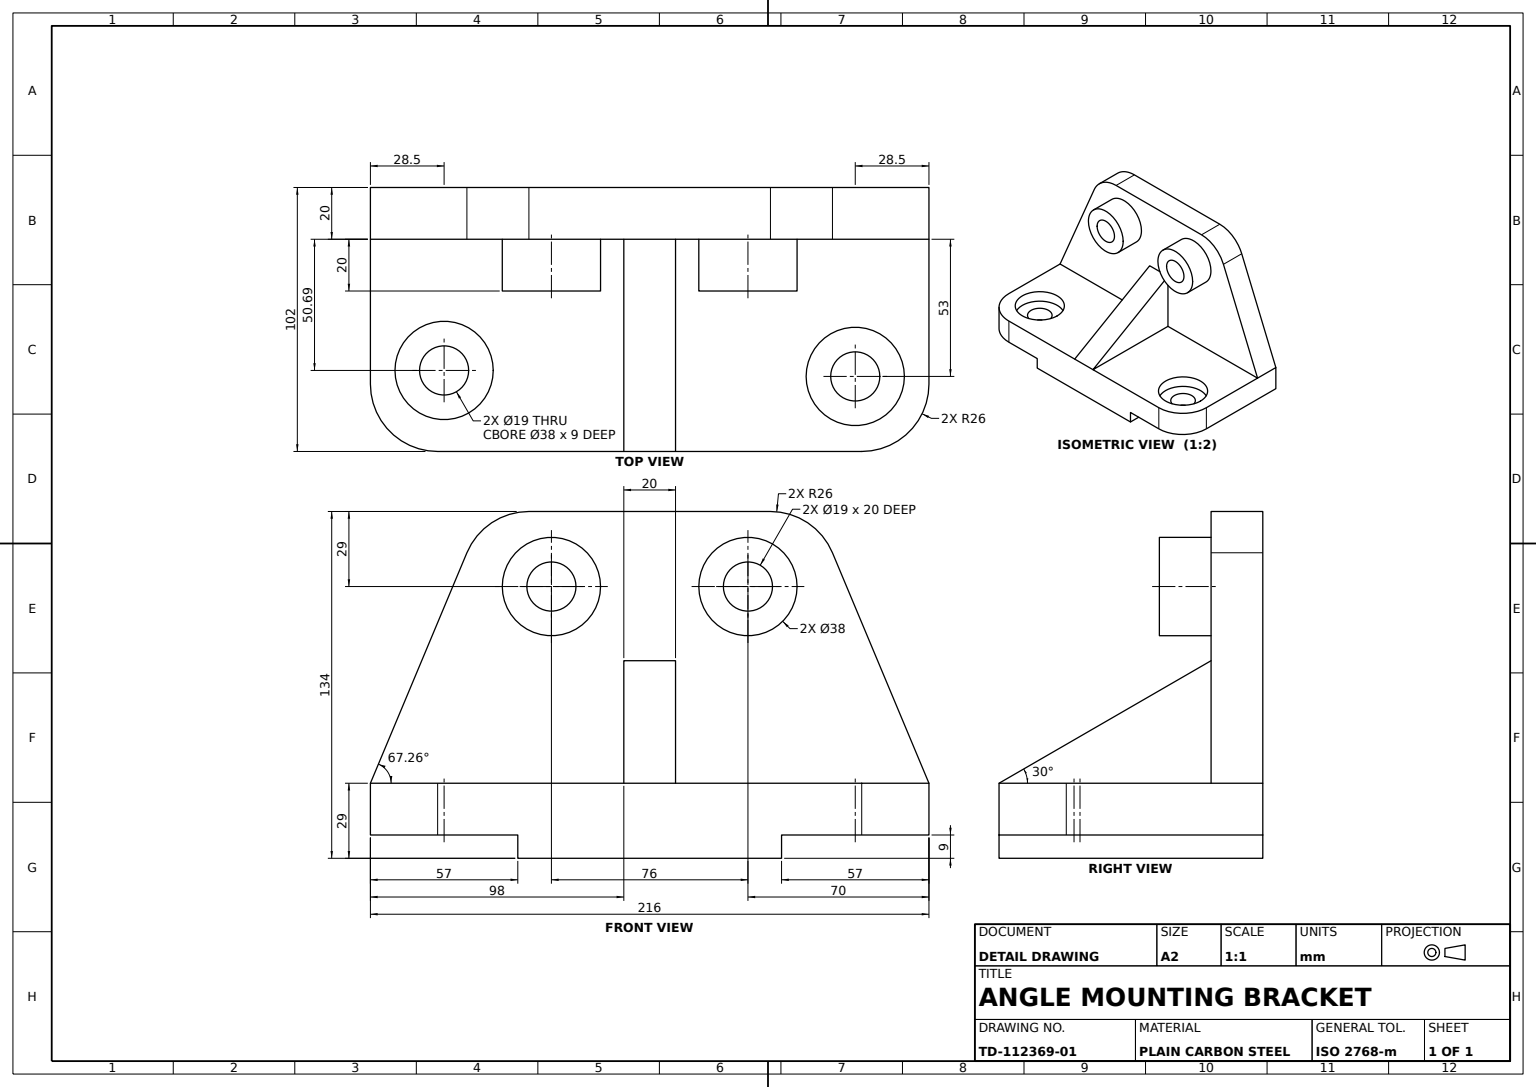
SolidWorks part; units mm, degrees
material "Plain Carbon Steel"
ref_plane "Front Plane" through (0, 0, 0) normal (0, 0, 1) x (1, 0, 0)
ref_plane "Top Plane" through (0, 0, 0) normal (0, 1, 0) x (1, 0, 0)
ref_plane "Right Plane" through (0, 0, 0) normal (1, 0, 0) x (0, 0, -1)
sketch "Base Plate Profile" plane through (0, 0, 0) normal (1, 0, 0) x (0, 0, -1)
  line L0 (0, 0) -> (57, 0)
  line L1 (57, 0) -> (57, -9)
  line L2 (57, -9) -> (159, -9)
  line L3 (159, -9) -> (159, 0)
  line L4 (159, 0) -> (216, 0)
  line L5 (216, 0) -> (216, 20)
  line L6 (216, 20) -> (0, 20)
  line L7 (0, 20) -> (0, 0)
  dimension "D1" = 57
  dimension "D2" = 9
  dimension "D3" = 102
  dimension "D4" = 216
  dimension "D5" = 20
extrude "Base Plate" add sketch "Base Plate Profile" along normal blind 102
ref_plane "Plane1" through (0, 0, 0) normal (1, 0, 0) x (0, 0, -1)
sketch "Upright Plate Profile" plane through (0, 0, 0) normal (1, 0, 0) x (0, 0, -1)
  line L0 (0, 20) -> (216, 20)
  line L2 (44, 125) -> (172, 125)
  line L4 (172, 125) -> (216, 20)
  line L5 (44, 125) -> (0, 20)
  dimension "D1" = 128
  dimension "D2" = 125
  dimension "D3" = 44
extrude "Upright Plate" add sketch "Upright Plate Profile" along normal blind 20
sketch "Upright Boss 1 Profile" plane through (20, 0, 0) normal (1, 0, 0) x (0, 0, -1)
  line L0 (172, 125) -> (44, 125) construction
  circle A0 centre (70, 96) radius 19
  circle A1 centre (70, 96) radius 9.5
  point P6 (108, 125)
  dimension "D1" = 76
  dimension "D3" = 19
  dimension "D4" = 38
  dimension "D2" = 38
extrude "Upright Boss 1" add sketch "Upright Boss 1 Profile" along normal blind 20
sketch "Upright Boss 2 Profile" plane through (20, 0, 0) normal (1, 0, 0) x (0, 0, -1)
  line L0 (0, 20) -> (216, 20) construction
  line L1 (172, 125) -> (44, 125) construction
  circle A0 centre (146, 96) radius 19
  circle A1 centre (146, 96) radius 9.5
  point P7 (108, 125)
  dimension "D1" = 76
  dimension "D3" = 19
  dimension "D4" = 38
  dimension "D2" = 38
extrude "Upright Boss 2" add sketch "Upright Boss 2 Profile" along normal blind 20
sketch "Base Pocket 1 Profile" plane through (0, 20, 0) normal (0, 1, 0) x (1, 0, 0)
  line L0 (102, 108) -> (102, 187.5) construction
  line L1 (102, 216) -> (102, 0) construction
  line L2 (102, 187.5) -> (73, 187.5) construction
  line L3 (73, 187.5) -> (73, 0) construction
  line L4 (102, 0) -> (20, 0) construction
  line L5 (102, 108) -> (102, 28.5) construction
  line L6 (102, 28.5) -> (73, 28.5) construction
  line L7 (20, 0) -> (20, 216) construction
  circle A0 centre (73, 187.5) radius 19
  dimension "D1" = 38
  dimension "D2" = 53
  dimension "D3" = 28.5
extrude "Base Pocket 1" cut sketch "Base Pocket 1 Profile" against normal blind 9
sketch "Mounting Hole 1 Profile" plane through (0, 11, 0) normal (0, 1, 0) x (1, 0, 0)
  circle A0 centre (73, 187.5) radius 9.5
  dimension "D1" = 19
extrude "Mounting Hole 1" cut sketch "Mounting Hole 1 Profile" against normal through all
sketch "Base Pocket 2 Profile" plane through (0, 20, 0) normal (0, 1, 0) x (1, 0, 0)
  line L0 (102, 108) -> (102, 28.5) construction
  line L1 (102, 216) -> (102, 0) construction
  line L2 (102, 28.5) -> (70.69, 28.5) construction
  line L3 (20, 0) -> (20, 216) construction
  circle A0 centre (70.69, 28.5) radius 19
  dimension "D1" = 38
  dimension "D2" = 50.69
  dimension "D3" = 28.5
extrude "Base Pocket 2" cut sketch "Base Pocket 2 Profile" against normal blind 9
sketch "Mounting Hole 2 Profile" plane through (0, 11, 0) normal (0, 1, 0) x (1, 0, 0)
  circle A0 centre (70.69, 28.5) radius 9.5
  dimension "D1" = 19
extrude "Mounting Hole 2" cut sketch "Mounting Hole 2 Profile" against normal through all
fillet "Upright Corner Fillet R26 1" radius 26 1 edges at (10, 125, -44)
fillet "Upright Corner Fillet R26 2" radius 26 1 edges at (10, 125, -172)
fillet "Base Corner Fillets R26" radius 26 2 edges at (102, 10, -216) (102, 10, 0)
ref_plane "Plane2" through (0, 0, -108) normal (0, 0, 1) x (1, 0, 0)
sketch "Gusset Rib Profile 30deg" plane through (0, 0, -108) normal (0, 0, 1) x (1, 0, 0)
  line L0 (102, 20) -> (20, 67.3427)
  line L1 (20, 109.0486) -> (20, 20) construction
  line L2 (102, 20) -> (76, 20) construction
  dimension "D1" = 30
rib "Gusset Rib" sketch "Gusset Rib Profile 30deg" sketch "Gusset Rib Profile 30deg" thickness 20 extrusion direction parallel to sketch draft on no parameters "D1"=20
